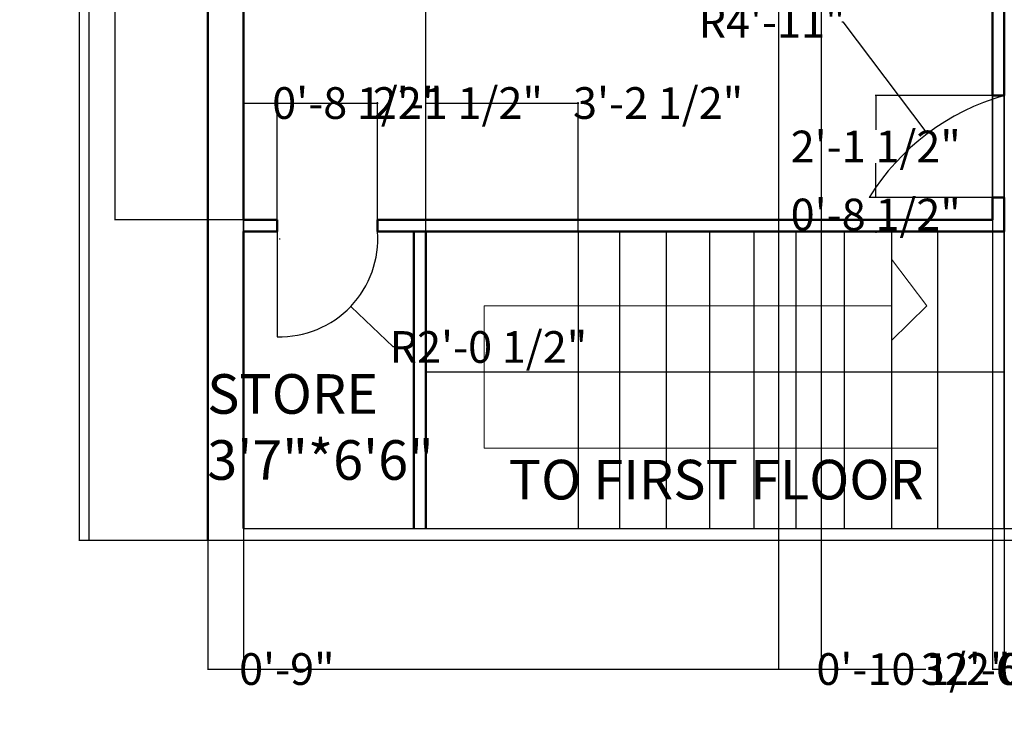
# Model space of a CAD drawing. Units: inches. Extents: x 3437 to 3994, y 3379 to 4084.
# Tile 1 of 6: x 3473 to 3722, y 3379 to 3555. Entities that reach past the tile are written whole.
import ezdxf

# ---------------------------------------------------------------- set-up
doc = ezdxf.new("R2010")
doc.units = ezdxf.units.IN
doc.header["$MEASUREMENT"] = 0
for name, color, linetype, lineweight in [('A-ANNO-DIMS', 2, 'Continuous', 18), ('A-ANNO-SYMB', 7, 'Continuous', 18), ('A-ANNO-TEXT', 7, 'Continuous', 18), ('A-AREA-IDEN', 7, 'Continuous', 25), ('A-DOOR', 3, 'Continuous', 25), ('A-FLOR-STRS', 7, 'Continuous', 25), ('A-WALL', 7, 'Continuous', 50), ('C-PROP', 3, 'Continuous', 25)]:
    doc.layers.add(name, color=color, linetype=linetype, lineweight=lineweight)
doc.styles.get("Standard").update_dxf_attribs({"font": 'arial.ttf'})
doc.dimstyles.get("Standard").update_dxf_attribs({"dimtxt": 8, "dimasz": 0.18, "dimexe": 0.18, "dimexo": 0.0625, "dimgap": 0.09, "dimtad": 0, "dimtih": 1, "dimtoh": 1, "dimdec": 0, "dimzin": 0, "dimdsep": 46, "dimlunit": 3, "dimtxsty": 'Standard', "dimcen": 0.09, "dimadec": 0, "dimazin": 0, "dimtfac": 1, "dimtdec": 0, "dimtofl": 0, "dimtmove": 0, "dimatfit": 3, "dimfxl": 1, "dimtolj": 1, "dimtzin": 0, "dimarcsym": 0})

# ---------------------------------------------------------------- blocks, each defined once
blk = doc.blocks.new('*D27')
at = {"layer": 'A-ANNO-DIMS', "color": 0, "lineweight": -2, "transparency": 16777216}
for p, q in [((3521.02, 3423.57), (3521.02, 3391.01)), ((3911.02, 3423.57), (3911.02, 3391.01)), ((3521.2, 3391.19), (3702.2, 3391.19)), ((3910.84, 3391.19), (3729.85, 3391.19))]:
    blk.add_line(p, q, dxfattribs=at)
at = {"layer": 'A-ANNO-DIMS', "color": 0, "transparency": 16777216}
for points in [[(3521.2, 3391.22), (3521.2, 3391.16), (3521.02, 3391.19)], [(3910.84, 3391.22), (3910.84, 3391.16), (3911.02, 3391.19)]]:
    blk.add_solid(points, dxfattribs=at)
at = {"layer": 'Defpoints', "color": 0, "transparency": 16777216}
for p in [(3521.02, 3423.64), (3911.02, 3423.64), (3911.02, 3391.19)]:
    blk.add_point(p, dxfattribs=at)
at = {"layer": 'A-ANNO-DIMS', "color": 0, "transparency": 16777216, "insert": (3716.02, 3391.19), "char_height": 8, "attachment_point": 5}
blk.add_mtext('\\A1;32\'-6"', dxfattribs=at)
blk = doc.blocks.new('*D28')
at = {"layer": 'A-ANNO-DIMS', "color": 0, "lineweight": -2, "transparency": 16777216}
for p, q in [((3520.96, 3993.64), (3488.39, 3993.64)), ((3488.57, 3993.46), (3488.57, 3712.81)), ((3488.57, 3423.82), (3488.57, 3704.46)), ((3520.96, 3423.64), (3488.39, 3423.64))]:
    blk.add_line(p, q, dxfattribs=at)
at = {"layer": 'A-ANNO-DIMS', "color": 0, "transparency": 16777216}
for points in [[(3488.54, 3993.46), (3488.6, 3993.46), (3488.57, 3993.64)], [(3488.54, 3423.82), (3488.6, 3423.82), (3488.57, 3423.64)]]:
    blk.add_solid(points, dxfattribs=at)
at = {"layer": 'Defpoints', "color": 0, "transparency": 16777216}
for p in [(3488.57, 3993.64), (3521.02, 3993.64), (3521.02, 3423.64)]:
    blk.add_point(p, dxfattribs=at)
at = {"layer": 'A-ANNO-DIMS', "color": 0, "transparency": 16777216, "insert": (3488.57, 3708.64), "char_height": 8, "attachment_point": 5}
blk.add_mtext('\\A1;47\'-6"', dxfattribs=at)
blk = doc.blocks.new('*D46')
at = {"layer": 'A-ANNO-DIMS', "color": 0, "lineweight": -2, "transparency": 16777216}
for p, q in [((3576.02, 3426.7), (3576.02, 4056.27)), ((3576.2, 4056.09), (3635.57, 4056.09)), ((3721.84, 4056.09), (3662.48, 4056.09)), ((3722.02, 3426.7), (3722.02, 4056.27))]:
    blk.add_line(p, q, dxfattribs=at)
at = {"layer": 'A-ANNO-DIMS', "color": 0, "transparency": 16777216}
for points in [[(3576.2, 4056.12), (3576.2, 4056.06), (3576.02, 4056.09)], [(3721.84, 4056.12), (3721.84, 4056.06), (3722.02, 4056.09)]]:
    blk.add_solid(points, dxfattribs=at)
at = {"layer": 'Defpoints', "color": 0, "transparency": 16777216}
for p in [(3722.02, 4056.09), (3576.02, 3426.64), (3722.02, 3426.64)]:
    blk.add_point(p, dxfattribs=at)
at = {"layer": 'A-ANNO-DIMS', "color": 0, "transparency": 16777216, "insert": (3649.02, 4056.09), "char_height": 8, "attachment_point": 5}
blk.add_mtext('\\A1;12\'-2"', dxfattribs=at)
blk = doc.blocks.new('*D47')
at = {"layer": 'A-ANNO-DIMS', "color": 0, "lineweight": -2, "transparency": 16777216}
for p, q in [((3521.02, 3993.57), (3521.02, 3391.01)), ((3530.02, 3984.57), (3530.02, 3391.01)), ((3521.2, 3391.19), (3529.84, 3391.19)), ((3530.02, 3391.19), (3530.2, 3391.19))]:
    blk.add_line(p, q, dxfattribs=at)
at = {"layer": 'A-ANNO-DIMS', "color": 0, "transparency": 16777216}
for points in [[(3521.2, 3391.22), (3521.2, 3391.16), (3521.02, 3391.19)], [(3529.84, 3391.22), (3529.84, 3391.16), (3530.02, 3391.19)]]:
    blk.add_solid(points, dxfattribs=at)
at = {"layer": 'Defpoints', "color": 0, "transparency": 16777216}
for p in [(3521.02, 3993.64), (3530.02, 3984.64), (3530.02, 3391.19)]:
    blk.add_point(p, dxfattribs=at)
at = {"layer": 'A-ANNO-DIMS', "color": 0, "transparency": 16777216, "insert": (3540.93, 3391.19), "char_height": 8, "attachment_point": 5}
blk.add_mtext('\\A1;0\'-9"', dxfattribs=at)
blk = doc.blocks.new('*D48')
at = {"layer": 'A-ANNO-DIMS', "color": 0, "lineweight": -2, "transparency": 16777216}
for p, q in [((3722.02, 3861.57), (3722.02, 3391.01)), ((3719.02, 3858.57), (3719.02, 3391.01)), ((3719.2, 3391.19), (3721.84, 3391.19)), ((3722.02, 3391.19), (3722.2, 3391.19))]:
    blk.add_line(p, q, dxfattribs=at)
at = {"layer": 'A-ANNO-DIMS', "color": 0, "transparency": 16777216}
for points in [[(3719.2, 3391.22), (3719.2, 3391.16), (3719.02, 3391.19)], [(3721.84, 3391.22), (3721.84, 3391.16), (3722.02, 3391.19)]]:
    blk.add_solid(points, dxfattribs=at)
at = {"layer": 'Defpoints', "color": 0, "transparency": 16777216}
for p in [(3722.02, 3861.64), (3719.02, 3858.64), (3722.02, 3391.19)]:
    blk.add_point(p, dxfattribs=at)
at = {"layer": 'A-ANNO-DIMS', "color": 0, "transparency": 16777216, "insert": (3732.93, 3391.19), "char_height": 8, "attachment_point": 5}
blk.add_mtext('\\A1;0\'-3"', dxfattribs=at)
blk = doc.blocks.new('*D49')
at = {"layer": 'A-ANNO-DIMS', "color": 0, "lineweight": -2, "transparency": 16777216}
for p, q in [((3530.02, 3504.7), (3530.02, 4056.27)), ((3530.2, 4056.09), (3611.07, 4056.09)), ((3718.84, 4056.09), (3637.98, 4056.09)), ((3719.02, 3504.7), (3719.02, 4056.27))]:
    blk.add_line(p, q, dxfattribs=at)
at = {"layer": 'A-ANNO-DIMS', "color": 0, "transparency": 16777216}
for points in [[(3530.2, 4056.12), (3530.2, 4056.06), (3530.02, 4056.09)], [(3718.84, 4056.12), (3718.84, 4056.06), (3719.02, 4056.09)]]:
    blk.add_solid(points, dxfattribs=at)
at = {"layer": 'Defpoints', "color": 0, "transparency": 16777216}
for p in [(3719.02, 4056.09), (3530.02, 3504.64), (3719.02, 3504.64)]:
    blk.add_point(p, dxfattribs=at)
at = {"layer": 'A-ANNO-DIMS', "color": 0, "transparency": 16777216, "insert": (3624.52, 4056.09), "char_height": 8, "attachment_point": 5}
blk.add_mtext('\\A1;15\'-9"', dxfattribs=at)
blk = doc.blocks.new('*D50')
at = {"layer": 'A-ANNO-DIMS', "color": 0, "lineweight": -2, "transparency": 16777216}
for p, q in [((3529.96, 3663.64), (3497.39, 3663.64)), ((3497.57, 3663.46), (3497.57, 3588.31)), ((3497.57, 3504.82), (3497.57, 3579.96)), ((3529.96, 3504.64), (3497.39, 3504.64))]:
    blk.add_line(p, q, dxfattribs=at)
at = {"layer": 'A-ANNO-DIMS', "color": 0, "transparency": 16777216}
for points in [[(3497.54, 3663.46), (3497.6, 3663.46), (3497.57, 3663.64)], [(3497.54, 3504.82), (3497.6, 3504.82), (3497.57, 3504.64)]]:
    blk.add_solid(points, dxfattribs=at)
at = {"layer": 'Defpoints', "color": 0, "transparency": 16777216}
for p in [(3497.57, 3663.64), (3530.02, 3663.64), (3530.02, 3504.64)]:
    blk.add_point(p, dxfattribs=at)
at = {"layer": 'A-ANNO-DIMS', "color": 0, "transparency": 16777216, "insert": (3497.57, 3584.14), "char_height": 8, "attachment_point": 5}
blk.add_mtext('\\A1;13\'-3"', dxfattribs=at)
blk = doc.blocks.new('*D62')
at = {"layer": 'A-ANNO-DIMS', "color": 0, "lineweight": -2, "transparency": 16777216}
for p, q in [((3721.96, 3535.98), (3689.39, 3535.98)), ((3689.57, 3535.8), (3689.57, 3527.35)), ((3689.57, 3510.44), (3689.57, 3518.9)), ((3721.96, 3510.26), (3689.39, 3510.26))]:
    blk.add_line(p, q, dxfattribs=at)
at = {"layer": 'A-ANNO-DIMS', "color": 0, "transparency": 16777216}
for points in [[(3689.54, 3535.8), (3689.6, 3535.8), (3689.57, 3535.98)], [(3689.54, 3510.44), (3689.6, 3510.44), (3689.57, 3510.26)]]:
    blk.add_solid(points, dxfattribs=at)
at = {"layer": 'Defpoints', "color": 0, "transparency": 16777216}
for p in [(3689.57, 3535.98), (3722.02, 3535.98), (3722.02, 3510.26)]:
    blk.add_point(p, dxfattribs=at)
at = {"layer": 'A-ANNO-DIMS', "color": 0, "transparency": 16777216, "insert": (3689.57, 3523.12), "char_height": 8, "attachment_point": 5}
blk.add_mtext('\\A1;2\'-1 1/2"', dxfattribs=at)
blk = doc.blocks.new('*D63')
at = {"layer": 'A-ANNO-DIMS', "color": 0, "lineweight": -2, "transparency": 16777216}
for p, q in [((3538.47, 3501.7), (3538.47, 3534.27)), ((3563.81, 3501.7), (3563.81, 3534.27)), ((3538.65, 3534.09), (3563.63, 3534.09)), ((3563.81, 3534.09), (3563.99, 3534.09))]:
    blk.add_line(p, q, dxfattribs=at)
at = {"layer": 'A-ANNO-DIMS', "color": 0, "transparency": 16777216}
for points in [[(3538.65, 3534.12), (3538.65, 3534.06), (3538.47, 3534.09)], [(3563.63, 3534.12), (3563.63, 3534.06), (3563.81, 3534.09)]]:
    blk.add_solid(points, dxfattribs=at)
at = {"layer": 'Defpoints', "color": 0, "transparency": 16777216}
for p in [(3563.81, 3534.09), (3538.47, 3501.64), (3563.81, 3501.64)]:
    blk.add_point(p, dxfattribs=at)
at = {"layer": 'A-ANNO-DIMS', "color": 0, "transparency": 16777216, "insert": (3584.1, 3534.09), "char_height": 8, "attachment_point": 5}
blk.add_mtext('\\A1;2\'-1 1/2"', dxfattribs=at)
blk = doc.blocks.new('*D69')
at = {"layer": 'A-ANNO-DIMS', "color": 0, "lineweight": -2, "transparency": 16777216}
for p, q in [((3576.02, 3501.7), (3576.02, 3534.27)), ((3614.42, 3501.7), (3614.42, 3534.27)), ((3576.2, 3534.09), (3614.24, 3534.09)), ((3614.42, 3534.09), (3614.6, 3534.09))]:
    blk.add_line(p, q, dxfattribs=at)
at = {"layer": 'A-ANNO-DIMS', "color": 0, "transparency": 16777216}
for points in [[(3576.2, 3534.12), (3576.2, 3534.06), (3576.02, 3534.09)], [(3614.24, 3534.12), (3614.24, 3534.06), (3614.42, 3534.09)]]:
    blk.add_solid(points, dxfattribs=at)
at = {"layer": 'Defpoints', "color": 0, "transparency": 16777216}
for p in [(3614.42, 3534.09), (3576.02, 3501.64), (3614.42, 3501.64)]:
    blk.add_point(p, dxfattribs=at)
at = {"layer": 'A-ANNO-DIMS', "color": 0, "transparency": 16777216, "insert": (3634.64, 3534.09), "char_height": 8, "attachment_point": 5}
blk.add_mtext('\\A1;3\'-2 1/2"', dxfattribs=at)
blk = doc.blocks.new('*D76')
at = {"layer": 'A-ANNO-DIMS', "color": 0, "lineweight": -2, "transparency": 16777216}
for p, q in [((3721.96, 3510.26), (3689.39, 3510.26)), ((3689.57, 3510.44), (3689.57, 3510.62)), ((3721.96, 3501.64), (3689.39, 3501.64)), ((3689.57, 3501.46), (3689.57, 3501.28))]:
    blk.add_line(p, q, dxfattribs=at)
at = {"layer": 'A-ANNO-DIMS', "color": 0, "transparency": 16777216}
for points in [[(3689.54, 3510.44), (3689.6, 3510.44), (3689.57, 3510.26)], [(3689.54, 3501.46), (3689.6, 3501.46), (3689.57, 3501.64)]]:
    blk.add_solid(points, dxfattribs=at)
at = {"layer": 'Defpoints', "color": 0, "transparency": 16777216}
for p in [(3689.57, 3510.26), (3722.02, 3510.26), (3722.02, 3501.64)]:
    blk.add_point(p, dxfattribs=at)
at = {"layer": 'A-ANNO-DIMS', "color": 0, "transparency": 16777216, "insert": (3689.57, 3505.95), "char_height": 8, "attachment_point": 5}
blk.add_mtext('\\A1;0\'-8 1/2"', dxfattribs=at)
blk = doc.blocks.new('*D77')
at = {"layer": 'A-ANNO-DIMS', "color": 0, "lineweight": -2, "transparency": 16777216}
for p, q in [((3530.02, 3501.7), (3530.02, 3534.27)), ((3538.47, 3501.7), (3538.47, 3534.27)), ((3530.2, 3534.09), (3538.29, 3534.09)), ((3538.47, 3534.09), (3538.65, 3534.09))]:
    blk.add_line(p, q, dxfattribs=at)
at = {"layer": 'A-ANNO-DIMS', "color": 0, "transparency": 16777216}
for points in [[(3530.2, 3534.12), (3530.2, 3534.06), (3530.02, 3534.09)], [(3538.29, 3534.12), (3538.29, 3534.06), (3538.47, 3534.09)]]:
    blk.add_solid(points, dxfattribs=at)
at = {"layer": 'Defpoints', "color": 0, "transparency": 16777216}
for p in [(3538.47, 3534.09), (3530.02, 3501.64), (3538.47, 3501.64)]:
    blk.add_point(p, dxfattribs=at)
at = {"layer": 'A-ANNO-DIMS', "color": 0, "transparency": 16777216, "insert": (3558.7, 3534.09), "char_height": 8, "attachment_point": 5}
blk.add_mtext('\\A1;0\'-8 1/2"', dxfattribs=at)
blk = doc.blocks.new('*D79')
at = {"layer": 'A-ANNO-DIMS', "color": 0, "lineweight": -2, "transparency": 16777216}
for p, q in [((3675.76, 3905.25), (3675.76, 3391.01)), ((3665.02, 3903.57), (3665.02, 3391.01)), ((3665.2, 3391.19), (3675.58, 3391.19)), ((3675.76, 3391.19), (3675.94, 3391.19))]:
    blk.add_line(p, q, dxfattribs=at)
at = {"layer": 'A-ANNO-DIMS', "color": 0, "transparency": 16777216}
for points in [[(3665.2, 3391.22), (3665.2, 3391.16), (3665.02, 3391.19)], [(3675.58, 3391.22), (3675.58, 3391.16), (3675.76, 3391.19)]]:
    blk.add_solid(points, dxfattribs=at)
at = {"layer": 'Defpoints', "color": 0, "transparency": 16777216}
for p in [(3675.76, 3905.31), (3665.02, 3903.64), (3675.76, 3391.19)]:
    blk.add_point(p, dxfattribs=at)
at = {"layer": 'A-ANNO-DIMS', "color": 0, "transparency": 16777216, "insert": (3699.09, 3391.19), "char_height": 8, "attachment_point": 5}
blk.add_mtext('\\A1;0\'-10 1/2"', dxfattribs=at)
blk = doc.blocks.new('*D88')
at = {"layer": 'A-ANNO-DIMS', "color": 0, "lineweight": -2, "transparency": 16777216}
for p, q in [((3681.05, 3554.61), (3681.23, 3554.61)), ((3681.23, 3554.61), (3702.45, 3526.46)), ((3738.02, 3479.16), (3738.2, 3479.16)), ((3738.11, 3479.07), (3738.11, 3479.25))]:
    blk.add_line(p, q, dxfattribs=at)
at = {"layer": 'A-ANNO-DIMS', "color": 0, "transparency": 16777216}
blk.add_solid([(3702.48, 3526.48), (3702.43, 3526.44), (3702.56, 3526.32)], dxfattribs=at)
at = {"layer": 'Defpoints', "color": 0, "transparency": 16777216}
for p in [(3702.56, 3526.32), (3738.11, 3479.16)]:
    blk.add_point(p, dxfattribs=at)
at = {"layer": 'A-ANNO-DIMS', "color": 0, "transparency": 16777216, "insert": (3663.39, 3554.61), "char_height": 8, "attachment_point": 5}
blk.add_mtext('\\A1;R4\'-11"', dxfattribs=at)
blk = doc.blocks.new('*D94')
at = {"layer": 'A-ANNO-DIMS', "color": 0, "lineweight": -2, "transparency": 16777216}
for p, q in [((3539.09, 3499.79), (3539.27, 3499.79)), ((3539.18, 3499.7), (3539.18, 3499.88)), ((3567.76, 3472.5), (3557.17, 3482.61)), ((3567.94, 3472.5), (3567.76, 3472.5))]:
    blk.add_line(p, q, dxfattribs=at)
at = {"layer": 'A-ANNO-DIMS', "color": 0, "transparency": 16777216}
blk.add_solid([(3557.19, 3482.63), (3557.15, 3482.59), (3557.04, 3482.73)], dxfattribs=at)
at = {"layer": 'Defpoints', "color": 0, "transparency": 16777216}
for p in [(3539.18, 3499.79), (3557.04, 3482.73)]:
    blk.add_point(p, dxfattribs=at)
at = {"layer": 'A-ANNO-DIMS', "color": 0, "transparency": 16777216, "insert": (3591.81, 3472.5), "char_height": 8, "attachment_point": 5}
blk.add_mtext('\\A1;R2\'-0 1/2"', dxfattribs=at)

msp = doc.modelspace()

# ---------------------------------------------------------------- linework, layer by layer
at = {"layer": 'A-ANNO-SYMB'}
for p, q in [((3702.51, 3482.89), (3693.52, 3494.67)), ((3590.73, 3446.95), (3590.73, 3482.89)), ((3590.73, 3482.89), (3693.52, 3482.89)), ((3702.51, 3482.89), (3693.52, 3474.16)), ((3705.15, 3446.95), (3590.73, 3446.95))]:
    msp.add_line(p, q, dxfattribs=at)
at = {"layer": 'A-DOOR'}
for p, q in [((3719.02, 3510.26), (3687.92, 3510.26)), ((3538.47, 3501.64), (3538.47, 3475.1))]:
    msp.add_line(p, q, dxfattribs=at)
for centre, radius, start, end in [((3738.11, 3479.16), 59.05, 105.8119, 148.2214), ((3539.18, 3499.79), 24.7, 268.3641, 4.2908)]:
    msp.add_arc(centre, radius, start, end, dxfattribs=at)
at = {"layer": 'A-FLOR-STRS'}
for p, q in [((3614.42, 3501.64), (3614.42, 3426.64)), ((3624.88, 3501.64), (3624.88, 3426.64)), ((3636.66, 3501.64), (3636.66, 3426.64)), ((3647.64, 3501.64), (3647.64, 3426.64)), ((3658.82, 3501.64), (3658.82, 3426.64)), ((3669.38, 3501.64), (3669.38, 3426.64)), ((3681.58, 3501.64), (3681.58, 3426.64)), ((3693.52, 3501.64), (3693.52, 3426.64)), ((3705.15, 3501.64), (3705.15, 3426.64)), ((3576.02, 3466.24), (3722.02, 3466.24))]:
    msp.add_line(p, q, dxfattribs=at)
at = {"layer": 'A-WALL'}
for p, q in [((3521.02, 3423.64), (3521.02, 3993.64)), ((3530.02, 3504.64), (3530.02, 3663.64)), ((3719.02, 3535.98), (3719.02, 3663.64)), ((3722.02, 3535.98), (3722.02, 3663.64)), ((3719.02, 3535.98), (3722.02, 3535.98)), ((3719.02, 3504.64), (3719.02, 3510.26)), ((3719.02, 3510.26), (3722.02, 3510.26)), ((3722.02, 3504.64), (3722.02, 3510.26)), ((3530.02, 3504.64), (3538.47, 3504.64)), ((3538.47, 3504.64), (3538.47, 3501.64)), ((3563.81, 3504.64), (3563.81, 3501.64)), ((3563.81, 3504.64), (3665.02, 3504.64)), ((3719.02, 3504.64), (3665.02, 3504.64)), ((3722.02, 3501.64), (3722.02, 3504.64)), ((3530.02, 3462.64), (3530.02, 3501.64)), ((3530.02, 3501.64), (3538.47, 3501.64)), ((3563.81, 3501.64), (3665.02, 3501.64)), ((3573.02, 3462.64), (3573.02, 3501.64)), ((3576.02, 3462.64), (3576.02, 3501.64)), ((3665.02, 3501.64), (3722.02, 3501.64)), ((3530.02, 3462.64), (3530.02, 3426.64)), ((3573.02, 3462.64), (3573.02, 3426.64)), ((3576.02, 3462.64), (3576.02, 3426.64))]:
    msp.add_line(p, q, dxfattribs=at)
at = {"layer": 'C-PROP'}
msp.add_line((3530.02, 3426.64), (3770.9, 3426.64), dxfattribs=at)
msp.add_lwpolyline([(3770.9, 3423.64), (3491.02, 3423.64), (3491.02, 4023.64), (3911.02, 4023.64), (3911.02, 3423.64), (3890.36, 3423.64)], dxfattribs=at)

# ---------------------------------------------------------------- texts
at = {"layer": 'A-ANNO-TEXT', "insert": (3596.94, 3444.01), "char_height": 10, "attachment_point": 1}
msp.add_mtext_dynamic_manual_height_columns('TO FIRST FLOOR', width=200.853, gutter_width=1, heights=[0], dxfattribs=at)
at = {"layer": 'A-AREA-IDEN', "insert": (3520.83, 3465.64), "char_height": 10, "attachment_point": 1}
msp.add_mtext_dynamic_manual_height_columns('STORE\\P3\'7"*6\'6"', width=200.853, gutter_width=1, heights=[0], dxfattribs=at)

# ---------------------------------------------------------------- dimensions: what is measured, and where the dimension line sits
at = {"layer": 'A-ANNO-DIMS'}
for base, p1, p2, picture, middle in [((3719.02, 4056.09), (3530.02, 3504.64), (3719.02, 3504.64), '*D49', (3624.52, 4056.09)), ((3722.02, 4056.09), (3576.02, 3426.64), (3722.02, 3426.64), '*D46', (3649.02, 4056.09)), ((3530.02, 3391.19), (3521.02, 3993.64), (3530.02, 3984.64), '*D47', (3540.93, 3391.19)), ((3675.76, 3391.19), (3665.02, 3903.64), (3675.76, 3905.31), '*D79', (3699.09, 3391.19)), ((3722.02, 3391.19), (3719.02, 3858.64), (3722.02, 3861.64), '*D48', (3732.93, 3391.19)), ((3538.4744, 3534.0859), (3530.0243, 3501.6359), (3538.4744, 3501.6359), '*D77', (3558.698, 3534.0859)), ((3614.42, 3534.09), (3576.02, 3501.64), (3614.42, 3501.64), '*D69', (3634.64, 3534.09)), ((3911.02, 3391.19), (3521.02, 3423.64), (3911.02, 3423.64), '*D27', (3716.02, 3391.19))]:
    dim = msp.add_linear_dim(base=base, p1=p1, p2=p2, dimstyle='Standard', override={"dimdec": 1, "dimlfac": 1, "dimrnd": 0, "dimzin": 1, "dimdsep": 46, "dimlunit": 4, "dimfrac": 2}, dxfattribs=at)
    dim.commit()
    dim.dimension.update_dxf_attribs({"geometry": picture, "text_midpoint": middle})
for base, p1, p2, angle, picture, middle in [((3488.57, 3993.64), (3521.02, 3423.64), (3521.02, 3993.64), 90, '*D28', (3488.57, 3708.64)), ((3497.57, 3663.64), (3530.02, 3504.64), (3530.02, 3663.64), 90, '*D50', (3497.57, 3584.14)), ((3563.81, 3534.09), (3538.47, 3501.64), (3563.81, 3501.64), 0, '*D63', (3584.1, 3534.09)), ((3689.57, 3535.98), (3722.02, 3510.26), (3722.02, 3535.98), 90, '*D62', (3689.57, 3523.12)), ((3689.57, 3510.26), (3722.02, 3501.64), (3722.02, 3510.26), 90, '*D76', (3689.57, 3505.95))]:
    dim = msp.add_linear_dim(base=base, p1=p1, p2=p2, angle=angle, dimstyle='Standard', override={"dimdec": 1, "dimlfac": 1, "dimrnd": 0, "dimzin": 1, "dimdsep": 46, "dimlunit": 4, "dimfrac": 2}, dxfattribs=at)
    dim.commit()
    dim.dimension.update_dxf_attribs({"geometry": picture, "text_midpoint": middle})
for center, mpoint, picture, middle in [((3738.11, 3479.16), (3702.56, 3526.32), '*D88', (3663.39, 3554.61)), ((3539.18, 3499.79), (3557.04, 3482.73), '*D94', (3591.81, 3472.5))]:
    dim = msp.add_radius_dim(center=center, mpoint=mpoint, dimstyle='Standard', override={"dimdec": 1, "dimlfac": 1, "dimrnd": 0, "dimzin": 1, "dimdsep": 46, "dimlunit": 4, "dimfrac": 2}, dxfattribs=at)
    dim.commit()
    dim.dimension.update_dxf_attribs({"geometry": picture, "text_midpoint": middle, "dimtype": 164})

doc.saveas('drawing.dxf')
